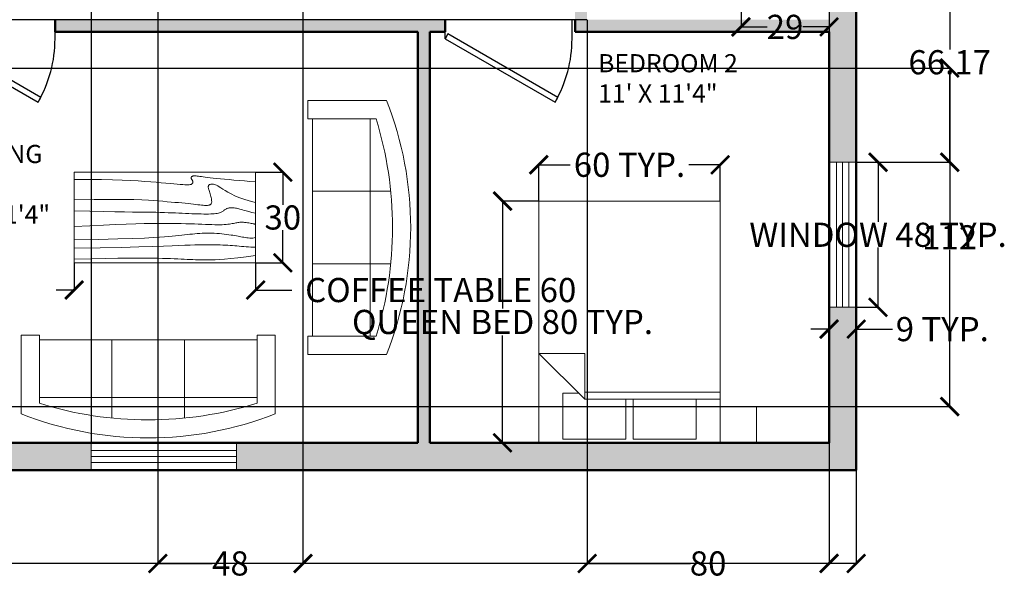
# Model space of a CAD drawing. Units: inches. Extents: x -30 to 744, y -375 to 57.
# Tile 6 of 8: x 355 to 680, y -375 to -190. Entities that reach past the tile are written whole.
import ezdxf

# ---------------------------------------------------------------- set-up
doc = ezdxf.new("R2010")
doc.units = ezdxf.units.IN
doc.header["$MEASUREMENT"] = 0
for name, color, linetype, lineweight in [('A-ANNO-DIMS', 2, 'Continuous', 18), ('A-AREA-IDEN', 7, 'Continuous', 25), ('A-DOOR', 3, 'Continuous', 25), ('A-FURN', 8, 'Continuous', 18), ('A-GLAZ', 4, 'Continuous', 18), ('A-WALL', 7, 'Continuous', 50)]:
    doc.layers.add(name, color=color, linetype=linetype, lineweight=lineweight)
doc.layers.add('A-WALL-PATT', color=251, linetype='Continuous', lineweight=13, true_color=0x636466)
doc.styles.get("Standard").update_dxf_attribs({"font": 'arial.ttf'})
doc.dimstyles.get("Standard").update_dxf_attribs({"dimtxt": 8, "dimasz": 6, "dimexe": 0.18, "dimexo": 0.0625, "dimgap": 0.09, "dimtad": 0, "dimtih": 1, "dimtoh": 1, "dimdec": 0, "dimzin": 0, "dimdsep": 46, "dimlunit": 4, "dimtxsty": 'Standard', "dimblk": 'ARCHTICK', "dimcen": 0.09, "dimadec": 0, "dimazin": 0, "dimtfac": 1, "dimtdec": 0, "dimtofl": 0, "dimtmove": 0, "dimatfit": 1, "dimldrblk": 'ARCHTICK', "dimfxl": 1, "dimtolj": 1, "dimtzin": 0, "dimarcsym": 0})

# ---------------------------------------------------------------- blocks, each defined once
blk = doc.blocks.new('*U4')
for p, q in [((0, 0), (0, 6)), ((40, 0), (40, 6))]:
    blk.add_line(p, q)
blk.add_lwpolyline([(0, 0), (34.64, -20), (35.52, -18.48), (0.87, 1.52)], close=True)
blk.add_arc((0, 0), 40, 330, 0)
blk = doc.blocks.new('*U3')
for p, q in [((0, 0), (0, 6)), ((40, 0), (40, 6))]:
    blk.add_line(p, q)
blk.add_lwpolyline([(0, 0), (34.64, -20), (35.52, -18.48), (0.88, 1.52)], close=True)
blk.add_arc((0, 0), 40, 330, 0)
blk = doc.blocks.new('Bed - Queen')
for p, q in [((0, -80.00003), (0, 0)), ((0, 0), (59.99999, 0)), ((59.99999, 0), (59.99999, -80.00003)), ((7.99999, -1.2), (28.79998, -1.2)), ((7.99999, -14.4), (7.99999, -1.2)), ((28.79998, -1.2), (28.79998, -14.4)), ((31.19999, -1.2), (51.99999, -1.2)), ((31.19999, -14.4), (31.19999, -1.2)), ((51.99999, -1.2), (51.99999, -16.4)), ((0, -14.4), (44.8, -14.4)), ((59.99999, -29.6), (44.8, -14.4)), ((44.8, -14.4), (44.8, -29.6)), ((44.8, -16.8), (0, -16.8)), ((51.99999, -16.4), (46.79936, -16.4)), ((44.8, -29.6), (59.99999, -29.6)), ((59.99999, -80.00003), (0, -80.00003))]:
    blk.add_line(p, q)
blk = doc.blocks.new('Sofa - Roundback 7 ft.')
for p, q in [((-12.00002, -32.4421), (-12.00003, -6.5971)), ((11.99997, -32.4421), (11.99998, -6.5971)), ((-36.000027, -34), (-36.000027, -11.4696)), ((35.99998, -34), (35.99998, -11.4696)), ((-35.999844, -13.3819), (35.9998, -13.3819)), ((-36.000027, -32.4421), (35.99998, -32.4421))]:
    blk.add_line(p, q)
for points in [[(-36.000027, -34), (-42.000027, -34), (-42.000027, -8)], [(41.99998, -8), (41.99998, -34), (35.99998, -34)]]:
    blk.add_lwpolyline(points)
for centre, radius, start, end in [((0, -114.25), 114.25, 68.43141, 111.5686), ((-0.00001, -127.1968), 121.1968, 72.72033, 107.2797)]:
    blk.add_arc(centre, radius, start, end)
blk = doc.blocks.new('Table - Rectangular Woodgrain 60 x 30 in.')
for p, q in [((0, 0), (0, -30)), ((60, 0), (0, 0)), ((60, -30), (60, 0)), ((0, -30), (60, -30))]:
    blk.add_line(p, q)
for points in [[(0, -2.4), (4.8155, -2.418), (9.0302, -2.4688), (12.709, -2.5477), (15.9167, -2.65), (18.7181, -2.7711), (21.1781, -2.9063), (23.3616, -3.0508), (25.3333, -3.2), (27.1477, -3.3495), (28.8172, -3.4958), (30.3437, -3.636), (31.7291, -3.7667), (32.9756, -3.8849), (34.0849, -3.9875), (35.059, -4.0714), (35.9, -4.1334), (36.6114, -4.1711), (37.2041, -4.1854), (37.6906, -4.1779), (38.0833, -4.15), (38.3948, -4.1034), (38.6375, -4.0396), (38.8239, -3.9602), (38.9666, -3.8667), (39.0764, -3.7608), (39.1573, -3.6448), (39.2116, -3.521), (39.2416, -3.3917), (39.2498, -3.2593), (39.2385, -3.1261), (39.21, -2.9944), (39.1666, -2.8667), (39.111, -2.7447), (39.0468, -2.6281), (38.978, -2.5163), (38.9083, -2.4083), (38.8418, -2.3035), (38.7823, -2.201), (38.7337, -2.1001), (38.7, -2), (38.6844, -1.9003), (38.6875, -1.8021), (38.7094, -1.707), (38.75, -1.6167), (38.8094, -1.5326), (38.8875, -1.4563), (38.9844, -1.3893), (39.1, -1.3333), (39.2351, -1.2896), (39.3937, -1.2583), (39.5804, -1.2396), (39.8, -1.2333), (40.057, -1.2396), (40.3562, -1.2583), (40.7023, -1.2896), (41.1, -1.3333), (41.5547, -1.3895), (42.0755, -1.4573), (42.6721, -1.5361), (43.3542, -1.625), (44.1316, -1.7233), (45.014, -1.8302), (46.0114, -1.9449), (47.1333, -2.0667), (48.3862, -2.1947), (49.7625, -2.3281), (51.2513, -2.4663), (52.8416, -2.6083), (54.5226, -2.7535), (56.2833, -2.9011), (58.1127, -3.0501), (60, -3.2)], [(0, -9.2), (6.5759, -9.0858), (11.9385, -9.0365), (16.2527, -9.0418), (19.6833, -9.0917), (22.3952, -9.1759), (24.5531, -9.2844), (26.322, -9.4069), (27.8666, -9.5333), (29.3241, -9.6553), (30.7203, -9.7719), (32.0532, -9.8837), (33.3208, -9.9917), (34.5213, -10.0965), (35.6526, -10.199), (36.7128, -10.2999), (37.7, -10.4), (38.6129, -10.4996), (39.4531, -10.5969), (40.223, -10.6895), (40.925, -10.775), (41.5613, -10.8512), (42.1344, -10.9156), (42.6465, -10.966), (43.1, -11), (43.4976, -11.0158), (43.8437, -11.0136), (44.143, -10.9942), (44.4, -10.9583), (44.6195, -10.9069), (44.8062, -10.8406), (44.9648, -10.7603), (45.1, -10.6667), (45.2155, -10.5598), (45.3114, -10.4365), (45.3871, -10.2929), (45.4416, -10.125), (45.4743, -9.929), (45.4844, -9.7011), (45.4709, -9.4371), (45.4333, -9.1333), (45.3716, -8.7883), (45.2896, -8.4104), (45.1919, -8.0107), (45.0833, -7.6), (44.9685, -7.1893), (44.8521, -6.7896), (44.7388, -6.4117), (44.6333, -6.0667), (44.54, -5.7628), (44.4614, -5.4979), (44.4001, -5.2675), (44.3583, -5.0667), (44.3384, -4.8909), (44.3427, -4.7354), (44.3736, -4.5956), (44.4333, -4.4667), (44.5236, -4.3453), (44.6427, -4.2333), (44.7884, -4.1339), (44.9583, -4.05), (45.1501, -3.9849), (45.3614, -3.9417), (45.59, -3.9234), (45.8333, -3.9333), (46.0915, -3.9749), (46.3734, -4.0531), (46.6906, -4.1736), (47.0542, -4.3417), (47.4756, -4.5629), (47.9661, -4.8427), (48.5372, -5.1866), (49.2, -5.6), (49.9676, -6.0844), (50.8594, -6.625), (51.8965, -7.2031), (53.1, -7.8), (54.491, -8.3969), (56.0906, -8.975), (57.9199, -9.5156), (60, -10)], [(0, -12.8), (5.1847, -12.9322), (9.6213, -13.0323), (13.3963, -13.1059), (16.5958, -13.1583), (19.3063, -13.1952), (21.614, -13.2219), (23.6054, -13.2439), (25.3666, -13.2667), (26.9728, -13.2947), (28.4531, -13.3281), (29.8256, -13.3663), (31.1083, -13.4083), (32.3191, -13.4535), (33.476, -13.501), (34.597, -13.5501), (35.7, -13.6), (36.7984, -13.6497), (37.8875, -13.6979), (38.9578, -13.743), (40, -13.7833), (41.0047, -13.8174), (41.9625, -13.8438), (42.864, -13.8607), (43.7, -13.8667), (44.4631, -13.8604), (45.1552, -13.8417), (45.7801, -13.8104), (46.3416, -13.7667), (46.8439, -13.7104), (47.2906, -13.6417), (47.6858, -13.5604), (48.0333, -13.4667), (48.3375, -13.3608), (48.6042, -13.2448), (48.8396, -13.121), (49.05, -12.9917), (49.2417, -12.8593), (49.4208, -12.7261), (49.5937, -12.5944), (49.7667, -12.4667), (49.9452, -12.3451), (50.1323, -12.2313), (50.3303, -12.1268), (50.5416, -12.0333), (50.7686, -11.9524), (51.0135, -11.8854), (51.2788, -11.8341), (51.5666, -11.8), (51.8785, -11.7843), (52.2116, -11.7865), (52.562, -11.8059), (52.926, -11.8417), (53.2998, -11.8931), (53.6795, -11.9594), (54.0614, -12.0397), (54.4416, -12.1333), (54.8223, -12.2401), (55.2293, -12.3625), (55.6942, -12.5037), (56.2489, -12.6667), (56.9251, -12.8547), (57.7545, -13.0708), (58.7689, -13.3182), (60, -13.6)], [(0, -18), (5.124, -17.7273), (9.6609, -17.5057), (13.6705, -17.3303), (17.2125, -17.1958), (20.3467, -17.0973), (23.1328, -17.0297), (25.6307, -16.9878), (27.9, -16.9667), (29.9928, -16.9617), (31.9302, -16.9703), (33.7254, -16.9907), (35.3917, -17.0208), (36.9423, -17.0588), (38.3906, -17.1026), (39.7499, -17.1503), (41.0333, -17.2), (42.2519, -17.2496), (43.4073, -17.2969), (44.4986, -17.3395), (45.525, -17.375), (46.4858, -17.4012), (47.3802, -17.4156), (48.2074, -17.416), (48.9667, -17.4), (49.6583, -17.3662), (50.2872, -17.3167), (50.8595, -17.2547), (51.3812, -17.1833), (51.8584, -17.1057), (52.2971, -17.025), (52.7034, -16.9443), (53.0833, -16.8667), (53.443, -16.7951), (53.789, -16.7313), (54.128, -16.6768), (54.4666, -16.6334), (54.8115, -16.6024), (55.1693, -16.5854), (55.5465, -16.5841), (55.95, -16.6), (56.3828, -16.6337), (56.8346, -16.6823), (57.2915, -16.7418), (57.7396, -16.8084), (58.165, -16.878), (58.5539, -16.9469), (58.8924, -17.0111), (59.1666, -17.0667), (59.3679, -17.1107), (59.5078, -17.1438), (59.6032, -17.1675), (59.6708, -17.1833), (59.7275, -17.193), (59.7901, -17.1979), (59.8753, -17.1998), (60, -17.2)], [(0, -22.4), (8.0098, -22.2501), (14.4094, -22.1011), (19.4168, -21.9535), (23.25, -21.8083), (26.1269, -21.6663), (28.2656, -21.5281), (29.884, -21.3947), (31.2, -21.2667), (32.3967, -21.1448), (33.5172, -21.0292), (34.5697, -20.9198), (35.5625, -20.8167), (36.5037, -20.7198), (37.4015, -20.6292), (38.2642, -20.5448), (39.1, -20.4667), (39.9164, -20.3951), (40.7187, -20.3313), (41.5117, -20.2768), (42.3, -20.2333), (43.0883, -20.2024), (43.8812, -20.1854), (44.6836, -20.1841), (45.5, -20.2), (46.3328, -20.234), (47.1747, -20.2844), (48.0163, -20.3488), (48.8479, -20.425), (49.66, -20.5106), (50.4429, -20.6031), (51.1872, -20.7004), (51.8833, -20.8), (52.5246, -20.8999), (53.1166, -20.9995), (53.6681, -21.0983), (54.1875, -21.1958), (54.6834, -21.2919), (55.1646, -21.3859), (55.6394, -21.4777), (56.1167, -21.5667), (56.6028, -21.6515), (57.0961, -21.7266), (57.5929, -21.7852), (58.0896, -21.8208), (58.5823, -21.8268), (59.0674, -21.7964), (59.5412, -21.723), (60, -21.6)], [(0, -25.2), (8.6355, -25.0504), (15.7026, -24.9031), (21.4049, -24.7606), (25.9458, -24.625), (29.529, -24.4988), (32.3578, -24.3844), (34.6359, -24.284), (36.5667, -24.2), (38.3213, -24.1341), (39.9417, -24.0854), (41.437, -24.0523), (42.8167, -24.0333), (44.0901, -24.0268), (45.2667, -24.0313), (46.3557, -24.0451), (47.3667, -24.0667), (48.309, -24.0947), (49.1928, -24.1287), (50.0284, -24.168), (50.826, -24.2125), (51.5959, -24.2617), (52.3483, -24.3151), (53.0935, -24.3725), (53.8417, -24.4334), (54.6009, -24.497), (55.3699, -24.561), (56.1454, -24.6226), (56.9239, -24.6792), (57.7021, -24.7279), (58.4764, -24.7662), (59.2435, -24.7911), (60, -24.8)], [(0, -28.8), (5.6867, -28.6681), (10.45, -28.5698), (14.407, -28.5012), (17.675, -28.4584), (20.3711, -28.4374), (22.6125, -28.4344), (24.5164, -28.4455), (26.2, -28.4667), (27.762, -28.4947), (29.2276, -28.5281), (30.6033, -28.5663), (31.8958, -28.6084), (33.1118, -28.6535), (34.2578, -28.7011), (35.3405, -28.7501), (36.3666, -28.8), (37.3443, -28.8497), (38.288, -28.8974), (39.2137, -28.9412), (40.1375, -28.9792), (41.0753, -29.0093), (42.0432, -29.0297), (43.0572, -29.0384), (44.1333, -29.0333), (45.2936, -29.0114), (46.5843, -28.9641), (48.0579, -28.8816), (49.7666, -28.7542), (51.7629, -28.5721), (54.0989, -28.3255), (56.8272, -28.0048), (60, -27.6)]]:
    blk.add_lwpolyline(points)
blk = doc.blocks.new('WIN-48IN')
for p, q in [((0, 0), (0, 48)), ((0, 48), (9, 48)), ((2.5, 48), (2.5, 0)), ((4.5, 48), (4.5, 0)), ((6.5, 48), (6.5, 0)), ((9, 48), (9, 0)), ((9, 48), (9, 0)), ((9, 0), (0, 0))]:
    blk.add_line(p, q)
blk = doc.blocks.new('NIGHTSTAND-12IN')
blk.add_lwpolyline([(0, 12), (0, 0), (12, 0), (12, 12)], close=True)
blk = doc.blocks.new('_ArchTick')
at = {"color": 0, "linetype": 'ByBlock', "const_width": 0.15}
blk.add_lwpolyline([(-0.5, -0.5), (0.5, 0.5)], dxfattribs=at)
blk = doc.blocks.new('*D26')
at = {"layer": 'A-ANNO-DIMS', "color": 0, "lineweight": -2, "transparency": 16777216}
for p, q in [((631.3, -237.46), (638.62, -237.46)), ((638.44, -237.46), (638.44, -257.23)), ((638.44, -285.46), (638.44, -265.69)), ((631.3, -285.46), (638.62, -285.46))]:
    blk.add_line(p, q, dxfattribs=at)
at = {"layer": 'Defpoints', "color": 0, "transparency": 16777216}
for p in [(631.24, -237.46), (638.44, -237.46), (631.24, -285.46)]:
    blk.add_point(p, dxfattribs=at)
at = {"layer": 'A-ANNO-DIMS', "color": 0, "lineweight": -2, "transparency": 16777216, "xscale": 6, "yscale": 6, "zscale": 6}
for p, rotation in [((638.44, -237.46), 90), ((638.44, -285.46), 270)]:
    blk.add_blockref('_ArchTick', p, dxfattribs=dict(at, rotation=rotation))
at = {"layer": 'A-ANNO-DIMS', "color": 0, "transparency": 16777216, "insert": (638.44, -261.46), "char_height": 8, "attachment_point": 5}
blk.add_mtext('\\A1;WINDOW 48 TYP.', dxfattribs=at)
blk = doc.blocks.new('*D27')
at = {"layer": 'A-ANNO-DIMS', "color": 0, "lineweight": -2, "transparency": 16777216}
for p, q in [((622.24, -285.53), (622.24, -292.84)), ((631.24, -285.53), (631.24, -292.84)), ((622.24, -292.66), (616.24, -292.66)), ((631.24, -292.66), (643.24, -292.66))]:
    blk.add_line(p, q, dxfattribs=at)
at = {"layer": 'Defpoints', "color": 0, "transparency": 16777216}
for p in [(622.24, -285.46), (631.24, -285.46), (631.24, -292.66)]:
    blk.add_point(p, dxfattribs=at)
at = {"layer": 'A-ANNO-DIMS', "color": 0, "lineweight": -2, "transparency": 16777216, "xscale": 6, "yscale": 6, "zscale": 6}
blk.add_blockref('_ArchTick', (622.24, -292.66), dxfattribs=at)
at = {"layer": 'A-ANNO-DIMS', "color": 0, "lineweight": -2, "transparency": 16777216, "xscale": 6, "yscale": 6, "zscale": 6, "rotation": 180}
blk.add_blockref('_ArchTick', (631.24, -292.66), dxfattribs=at)
at = {"layer": 'A-ANNO-DIMS', "color": 0, "transparency": 16777216, "insert": (659.69, -292.66), "char_height": 8, "attachment_point": 5}
blk.add_mtext('\\A1;9 TYP.', dxfattribs=at)
blk = doc.blocks.new('*D32')
at = {"layer": 'A-ANNO-DIMS', "color": 0, "lineweight": -2, "transparency": 16777216}
for p, q in [((526.17, -250.3), (514.06, -250.3)), ((514.24, -250.3), (514.24, -285.82)), ((514.24, -330.3), (514.24, -294.77)), ((526.17, -330.3), (514.06, -330.3))]:
    blk.add_line(p, q, dxfattribs=at)
at = {"layer": 'Defpoints', "color": 0, "transparency": 16777216}
for p in [(526.24, -250.3), (514.24, -330.3), (526.24, -330.3)]:
    blk.add_point(p, dxfattribs=at)
at = {"layer": 'A-ANNO-DIMS', "color": 0, "lineweight": -2, "transparency": 16777216, "xscale": 6, "yscale": 6, "zscale": 6}
for p, rotation in [((514.24, -250.3), 90), ((514.24, -330.3), 270)]:
    blk.add_blockref('_ArchTick', p, dxfattribs=dict(at, rotation=rotation))
at = {"layer": 'A-ANNO-DIMS', "color": 0, "transparency": 16777216, "insert": (514.24, -290.3), "char_height": 8, "attachment_point": 5}
blk.add_mtext('\\A1;QUEEN BED 80 TYP.', dxfattribs=at)
blk = doc.blocks.new('*D33')
at = {"layer": 'A-ANNO-DIMS', "color": 0, "lineweight": -2, "transparency": 16777216}
for p, q in [((526.24, -250.23), (526.24, -238.12)), ((526.24, -238.3), (536.65, -238.3)), ((586.24, -238.3), (575.82, -238.3)), ((586.24, -250.23), (586.24, -238.12))]:
    blk.add_line(p, q, dxfattribs=at)
at = {"layer": 'Defpoints', "color": 0, "transparency": 16777216}
for p in [(526.24, -238.3), (526.24, -250.3), (586.24, -250.3)]:
    blk.add_point(p, dxfattribs=at)
at = {"layer": 'A-ANNO-DIMS', "color": 0, "lineweight": -2, "transparency": 16777216, "xscale": 6, "yscale": 6, "zscale": 6, "rotation": 180.0000000000009}
blk.add_blockref('_ArchTick', (526.24, -238.3), dxfattribs=at)
at = {"layer": 'A-ANNO-DIMS', "color": 0, "lineweight": -2, "transparency": 16777216, "xscale": 6, "yscale": 6, "zscale": 6}
blk.add_blockref('_ArchTick', (586.24, -238.3), dxfattribs=at)
at = {"layer": 'A-ANNO-DIMS', "color": 0, "transparency": 16777216, "insert": (556.24, -238.3), "char_height": 8, "attachment_point": 5}
blk.add_mtext('\\A1;60 TYP.', dxfattribs=at)
blk = doc.blocks.new('*D37')
at = {"layer": 'A-ANNO-DIMS', "color": 0, "lineweight": -2, "transparency": 16777216}
for p, q in [((593.12, -185.47), (593.12, -192.86)), ((622.24, -185.47), (622.24, -192.86)), ((593.12, -192.68), (601.78, -192.68)), ((622.24, -192.68), (613.57, -192.68))]:
    blk.add_line(p, q, dxfattribs=at)
at = {"layer": 'Defpoints', "color": 0, "transparency": 16777216}
for p in [(593.12, -185.4), (622.24, -185.4), (622.24, -192.68)]:
    blk.add_point(p, dxfattribs=at)
at = {"layer": 'A-ANNO-DIMS', "color": 0, "lineweight": -2, "transparency": 16777216, "xscale": 6, "yscale": 6, "zscale": 6, "rotation": 180}
blk.add_blockref('_ArchTick', (593.12, -192.68), dxfattribs=at)
at = {"layer": 'A-ANNO-DIMS', "color": 0, "lineweight": -2, "transparency": 16777216, "xscale": 6, "yscale": 6, "zscale": 6}
blk.add_blockref('_ArchTick', (622.24, -192.68), dxfattribs=at)
at = {"layer": 'A-ANNO-DIMS', "color": 0, "transparency": 16777216, "insert": (607.68, -192.68), "char_height": 8, "attachment_point": 5}
blk.add_mtext('\\A1;29', dxfattribs=at)
blk = doc.blocks.new('*D58')
at = {"layer": 'A-ANNO-DIMS', "color": 0, "lineweight": -2, "transparency": 16777216}
for p, q in [((372.57, -270.8), (372.57, -279.92)), ((432.57, -270.8), (432.57, -279.92)), ((372.57, -279.74), (366.57, -279.74)), ((432.57, -279.74), (444.57, -279.74))]:
    blk.add_line(p, q, dxfattribs=at)
at = {"layer": 'Defpoints', "color": 0, "transparency": 16777216}
for p in [(372.57, -270.74), (432.57, -270.74), (432.57, -279.74)]:
    blk.add_point(p, dxfattribs=at)
at = {"layer": 'A-ANNO-DIMS', "color": 0, "lineweight": -2, "transparency": 16777216, "xscale": 6, "yscale": 6, "zscale": 6}
blk.add_blockref('_ArchTick', (372.57, -279.74), dxfattribs=at)
at = {"layer": 'A-ANNO-DIMS', "color": 0, "lineweight": -2, "transparency": 16777216, "xscale": 6, "yscale": 6, "zscale": 6, "rotation": 180}
blk.add_blockref('_ArchTick', (432.57, -279.74), dxfattribs=at)
at = {"layer": 'A-ANNO-DIMS', "color": 0, "transparency": 16777216, "insert": (493.8, -279.74), "char_height": 8, "attachment_point": 5}
blk.add_mtext('\\A1;COFFEE TABLE 60', dxfattribs=at)
blk = doc.blocks.new('*D59')
at = {"layer": 'A-ANNO-DIMS', "color": 0, "lineweight": -2, "transparency": 16777216}
for p, q in [((432.63, -240.74), (441.75, -240.74)), ((441.57, -240.74), (441.57, -251.56)), ((441.57, -270.74), (441.57, -259.91)), ((432.63, -270.74), (441.75, -270.74))]:
    blk.add_line(p, q, dxfattribs=at)
at = {"layer": 'Defpoints', "color": 0, "transparency": 16777216}
for p in [(432.57, -240.74), (441.57, -240.74), (432.57, -270.74)]:
    blk.add_point(p, dxfattribs=at)
at = {"layer": 'A-ANNO-DIMS', "color": 0, "lineweight": -2, "transparency": 16777216, "xscale": 6, "yscale": 6, "zscale": 6}
for p, rotation in [((441.57, -240.74), 90), ((441.57, -270.74), 270)]:
    blk.add_blockref('_ArchTick', p, dxfattribs=dict(at, rotation=rotation))
at = {"layer": 'A-ANNO-DIMS', "color": 0, "transparency": 16777216, "insert": (441.57, -255.74), "char_height": 8, "attachment_point": 5}
blk.add_mtext('\\A1;30', dxfattribs=at)
blk = doc.blocks.new('*D60')
at = {"layer": 'A-ANNO-DIMS', "color": 0, "lineweight": -2, "transparency": 16777216}
for p, q in [((31.24, -339.36), (31.24, -370.38)), ((631.24, -339.36), (631.24, -370.38)), ((31.24, -370.2), (322.3, -370.2)), ((631.24, -370.2), (340.17, -370.2))]:
    blk.add_line(p, q, dxfattribs=at)
at = {"layer": 'Defpoints', "color": 0, "transparency": 16777216}
for p in [(31.24, -339.3), (631.24, -339.3), (631.24, -370.2)]:
    blk.add_point(p, dxfattribs=at)
at = {"layer": 'A-ANNO-DIMS', "color": 0, "lineweight": -2, "transparency": 16777216, "xscale": 6, "yscale": 6, "zscale": 6, "rotation": 180}
blk.add_blockref('_ArchTick', (31.24, -370.2), dxfattribs=at)
at = {"layer": 'A-ANNO-DIMS', "color": 0, "lineweight": -2, "transparency": 16777216, "xscale": 6, "yscale": 6, "zscale": 6}
blk.add_blockref('_ArchTick', (631.24, -370.2), dxfattribs=at)
at = {"layer": 'A-ANNO-DIMS', "color": 0, "transparency": 16777216, "insert": (331.24, -370.2), "char_height": 8, "attachment_point": 5}
blk.add_mtext('\\A1;600', dxfattribs=at)
blk = doc.blocks.new('*D62')
at = {"layer": 'A-ANNO-DIMS', "color": 0, "lineweight": -2, "transparency": 16777216}
for p, q in [((542.24, -190.36), (542.24, -370.38)), ((622.24, -190.36), (622.24, -370.38)), ((542.24, -370.2), (576.42, -370.2)), ((622.24, -370.2), (588.05, -370.2))]:
    blk.add_line(p, q, dxfattribs=at)
at = {"layer": 'Defpoints', "color": 0, "transparency": 16777216}
for p in [(542.24, -190.3), (622.24, -190.3), (622.24, -370.2)]:
    blk.add_point(p, dxfattribs=at)
at = {"layer": 'A-ANNO-DIMS', "color": 0, "lineweight": -2, "transparency": 16777216, "xscale": 6, "yscale": 6, "zscale": 6, "rotation": 180}
blk.add_blockref('_ArchTick', (542.24, -370.2), dxfattribs=at)
at = {"layer": 'A-ANNO-DIMS', "color": 0, "lineweight": -2, "transparency": 16777216, "xscale": 6, "yscale": 6, "zscale": 6}
blk.add_blockref('_ArchTick', (622.24, -370.2), dxfattribs=at)
at = {"layer": 'A-ANNO-DIMS', "color": 0, "transparency": 16777216, "insert": (582.24, -370.2), "char_height": 8, "attachment_point": 5}
blk.add_mtext('\\A1;80', dxfattribs=at)
blk = doc.blocks.new('*D63')
at = {"layer": 'A-ANNO-DIMS', "color": 0, "lineweight": -2, "transparency": 16777216}
for p, q in [((542.17, -132.3), (-16.61, -132.3)), ((-16.43, -132.3), (-16.43, -157.12)), ((-16.43, -190.3), (-16.43, -165.47)), ((542.17, -190.3), (-16.61, -190.3))]:
    blk.add_line(p, q, dxfattribs=at)
at = {"layer": 'Defpoints', "color": 0, "transparency": 16777216}
for p in [(-16.43, -132.3), (542.24, -132.3), (542.24, -190.3)]:
    blk.add_point(p, dxfattribs=at)
at = {"layer": 'A-ANNO-DIMS', "color": 0, "lineweight": -2, "transparency": 16777216, "xscale": 6, "yscale": 6, "zscale": 6}
for p, rotation in [((-16.43, -132.3), 90), ((-16.43, -190.3), 270)]:
    blk.add_blockref('_ArchTick', p, dxfattribs=dict(at, rotation=rotation))
at = {"layer": 'A-ANNO-DIMS', "color": 0, "transparency": 16777216, "insert": (-16.43, -161.3), "char_height": 8, "attachment_point": 5}
blk.add_mtext('\\A1;58', dxfattribs=at)
blk = doc.blocks.new('*D64')
at = {"layer": 'A-ANNO-DIMS', "color": 0, "lineweight": -2, "transparency": 16777216}
for p, q in [((40.3, -206.3), (662.32, -206.3)), ((662.14, -206.3), (662.14, -258.19)), ((662.14, -318.3), (662.14, -266.4)), ((40.3, -318.3), (662.32, -318.3))]:
    blk.add_line(p, q, dxfattribs=at)
at = {"layer": 'Defpoints', "color": 0, "transparency": 16777216}
for p in [(40.24, -206.3), (662.14, -206.3), (40.24, -318.3)]:
    blk.add_point(p, dxfattribs=at)
at = {"layer": 'A-ANNO-DIMS', "color": 0, "lineweight": -2, "transparency": 16777216, "xscale": 6, "yscale": 6, "zscale": 6}
for p, rotation in [((662.14, -206.3), 90), ((662.14, -318.3), 270)]:
    blk.add_blockref('_ArchTick', p, dxfattribs=dict(at, rotation=rotation))
at = {"layer": 'A-ANNO-DIMS', "color": 0, "transparency": 16777216, "insert": (662.14, -262.3), "char_height": 8, "attachment_point": 5}
blk.add_mtext('\\A1;112', dxfattribs=at)
blk = doc.blocks.new('*D74')
at = {"layer": 'A-ANNO-DIMS', "color": 0, "lineweight": -2, "transparency": 16777216}
for p, q in [((318.24, -330.23), (318.24, 51.78)), ((318.24, 51.6), (342.41, 51.6)), ((378.24, 51.6), (354.06, 51.6)), ((378.24, -330.23), (378.24, 51.78))]:
    blk.add_line(p, q, dxfattribs=at)
at = {"layer": 'Defpoints', "color": 0, "transparency": 16777216}
for p in [(378.24, 51.6), (318.24, -330.3), (378.24, -330.3)]:
    blk.add_point(p, dxfattribs=at)
at = {"layer": 'A-ANNO-DIMS', "color": 0, "lineweight": -2, "transparency": 16777216, "xscale": 6, "yscale": 6, "zscale": 6, "rotation": 180}
blk.add_blockref('_ArchTick', (318.24, 51.6), dxfattribs=at)
at = {"layer": 'A-ANNO-DIMS', "color": 0, "lineweight": -2, "transparency": 16777216, "xscale": 6, "yscale": 6, "zscale": 6}
blk.add_blockref('_ArchTick', (378.24, 51.6), dxfattribs=at)
at = {"layer": 'A-ANNO-DIMS', "color": 0, "transparency": 16777216, "insert": (348.24, 51.6), "char_height": 8, "attachment_point": 5}
blk.add_mtext('\\A1;60', dxfattribs=at)
blk = doc.blocks.new('*D78')
at = {"layer": 'A-ANNO-DIMS', "color": 0, "lineweight": -2, "transparency": 16777216}
for p, q in [((631.3, -171.3), (662.32, -171.3)), ((662.14, -171.3), (662.14, -200.21)), ((662.14, -237.46), (662.14, -208.55)), ((631.3, -237.46), (662.32, -237.46))]:
    blk.add_line(p, q, dxfattribs=at)
at = {"layer": 'Defpoints', "color": 0, "transparency": 16777216}
for p in [(631.24, -171.3), (662.14, -171.3), (631.24, -237.46)]:
    blk.add_point(p, dxfattribs=at)
at = {"layer": 'A-ANNO-DIMS', "color": 0, "lineweight": -2, "transparency": 16777216, "xscale": 6, "yscale": 6, "zscale": 6}
for p, rotation in [((662.14, -171.3), 90), ((662.14, -237.46), 270)]:
    blk.add_blockref('_ArchTick', p, dxfattribs=dict(at, rotation=rotation))
at = {"layer": 'A-ANNO-DIMS', "color": 0, "transparency": 16777216, "insert": (662.14, -204.38), "char_height": 8, "attachment_point": 5}
blk.add_mtext('\\A1;66.17', dxfattribs=at)
blk = doc.blocks.new('*D83')
at = {"layer": 'A-ANNO-DIMS', "color": 0, "lineweight": -2, "transparency": 16777216}
for p, q in [((400.24, -132.36), (400.24, -370.38)), ((448.24, -132.36), (448.24, -370.38)), ((400.24, -370.2), (418.25, -370.2)), ((448.24, -370.2), (430.22, -370.2))]:
    blk.add_line(p, q, dxfattribs=at)
at = {"layer": 'Defpoints', "color": 0, "transparency": 16777216}
for p in [(400.24, -132.3), (448.24, -132.3), (448.24, -370.2)]:
    blk.add_point(p, dxfattribs=at)
at = {"layer": 'A-ANNO-DIMS', "color": 0, "lineweight": -2, "transparency": 16777216, "xscale": 6, "yscale": 6, "zscale": 6, "rotation": 180}
blk.add_blockref('_ArchTick', (400.24, -370.2), dxfattribs=at)
at = {"layer": 'A-ANNO-DIMS', "color": 0, "lineweight": -2, "transparency": 16777216, "xscale": 6, "yscale": 6, "zscale": 6}
blk.add_blockref('_ArchTick', (448.24, -370.2), dxfattribs=at)
at = {"layer": 'A-ANNO-DIMS', "color": 0, "transparency": 16777216, "insert": (424.24, -370.2), "char_height": 8, "attachment_point": 5}
blk.add_mtext('\\A1;48', dxfattribs=at)

msp = doc.modelspace()

# ---------------------------------------------------------------- hatches: boundary and pattern name
at = {"layer": 'A-WALL-PATT'}
h = msp.add_hatch(color=256, dxfattribs=at)
h.dxf.hatch_style = 1
h.paths.add_polyline_path([(40.2356, 11.7031), (204.2356, 11.7031), (204.2356, -24.2969), (208.2356, -24.2969), (208.2356, 11.7031), (233.4275, 11.7031), (233.4275, 20.7031), (31.2356, 20.7031), (31.2356, -34.2969), (40.2356, -34.2969)])
h.paths.add_polyline_path([(40.2356, -82.2969), (31.2356, -82.2969), (31.2356, -132.2969), (40.2356, -132.2969), (51.0767, -132.2969), (111.3137, -132.2969), (111.3137, -143.2969), (120.3137, -143.2969), (120.3137, -132.2969), (156.2356, -132.2969), (156.2356, -128.2969), (113.6001, -128.2969), (113.6001, -128.3034), (53.6001, -128.3034), (40.2356, -128.2969)])
h.paths.add_polyline_path([(302.4681, 20.7031), (257.4275, 20.7031), (257.4275, 11.7031), (286.2356, 11.7031), (286.2356, -60.2969), (208.2356, -60.2969), (208.2356, -54.2969), (204.2356, -54.2969), (204.2356, -64.2969), (208.2356, -64.2969), (286.2356, -64.2969), (286.2356, -128.2969), (264.8954, -128.2969), (208.2356, -128.2969), (204.2356, -128.2969), (198.2356, -128.2969), (198.2356, -132.2969), (290.2356, -132.2969), (290.2356, -128.2969), (290.2356, 11.7031), (302.4681, 11.7031)])
h.paths.add_polyline_path([(405.515, 20.7031), (350.4681, 20.7031), (350.4681, 11.7031), (362.2356, 11.7031), (362.2356, -34.2969), (366.2356, -34.2969), (366.2356, 11.7031), (405.515, 11.7031)])
h.paths.add_polyline_path([(530.2713, 20.7031), (453.515, 20.7031), (453.515, 11.7031), (486.2356, 11.7031), (486.2356, -128.2969), (448.2356, -128.2969), (448.2356, -132.2969), (486.2356, -132.2969), (490.2356, -132.2969), (496.2356, -132.2969), (496.2356, -128.2969), (490.2356, -128.2969), (490.2356, 11.7031), (530.2713, 11.7031)])
h.paths.add_polyline_path([(631.2356, 20.7031), (578.2713, 20.7031), (578.2713, 11.7031), (622.2356, 11.7031), (622.2356, -37.4001), (631.2356, -37.4001)])
h.paths.add_polyline_path([(631.2356, -85.4001), (622.2356, -85.4001), (622.2356, -91.4001), (622.2356, -103.4001), (622.2356, -128.2969), (538.2356, -128.2969), (538.2356, -132.2969), (538.2356, -154.2969), (542.2356, -154.2969), (542.2356, -132.2969), (575.1375, -132.2969), (585.6313, -131.9348), (585.6438, -132.2969), (622.2356, -132.2969), (622.2356, -147.2969), (631.2356, -147.2969)])
h.paths.add_polyline_path([(631.2356, -171.2969), (622.2356, -171.2969), (622.2356, -185.4028), (622.2356, -186.2969), (622.2356, -190.2969), (542.2356, -190.2969), (542.2356, -184.2969), (538.2356, -184.2969), (538.2356, -190.2969), (538.2356, -194.2969), (622.2356, -194.2969), (622.2356, -237.4632), (631.2356, -237.4632)])
h.paths.add_polyline_path([(631.2356, -285.4632), (622.2356, -285.4632), (622.2356, -330.2969), (490.2356, -330.2969), (490.2356, -194.2969), (494.2356, -194.2969), (495.2356, -194.2969), (495.2356, -190.2969), (494.2356, -190.2969), (490.2356, -190.2969), (486.2356, -190.2969), (366.2356, -190.2969), (366.2356, -194.2969), (486.2356, -194.2969), (486.2356, -330.2969), (426.2356, -330.2969), (426.2356, -339.2969), (631.2356, -339.2969)])
h.paths.add_polyline_path([(378.2356, -330.2969), (318.2356, -330.2969), (318.2356, -194.2969), (324.2356, -194.2969), (324.2356, -190.2969), (318.2356, -190.2969), (314.2356, -190.2969), (314.2356, -194.2969), (314.2356, -330.2969), (278.2356, -330.2969), (278.2356, -339.2969), (378.2356, -339.2969)])
h.paths.add_polyline_path([(190.2356, -330.2969), (40.2356, -330.2969), (40.2356, -318.2969), (31.2356, -318.2969), (31.2356, -330.2969), (31.2356, -339.2969), (190.2356, -339.2969)])
h.paths.add_polyline_path([(230.2356, -330.2969), (194.2356, -330.2969), (194.2356, -194.2969), (194.2356, -190.2969), (190.2356, -190.2969), (184.2356, -190.2969), (184.2356, -194.2969), (190.2356, -194.2969), (190.2356, -339.2969), (230.2356, -339.2969)])
h.paths.add_polyline_path([(142.2356, -190.2969), (120.3137, -190.2969), (120.3137, -184.2969), (116.3137, -184.2969), (111.3137, -184.2969), (111.3137, -190.2969), (40.2356, -190.2969), (31.2356, -190.2969), (31.2356, -194.2969), (31.2356, -206.2969), (40.2356, -206.2969), (40.2356, -194.2969), (142.2356, -194.2969)])

# ---------------------------------------------------------------- linework, layer by layer
at = {"layer": 'A-WALL'}
for p, q in [((366.2356, -190.2969), (366.2356, -194.2969)), ((495.2356, -190.2969), (495.2356, -194.2969)), ((538.2356, -190.2969), (538.2356, -194.2969)), ((366.2356, -194.2969), (486.2356, -194.2969)), ((486.2356, -194.2969), (486.2356, -330.2969)), ((490.2356, -194.2969), (494.2356, -194.2969)), ((490.2356, -194.3643), (490.2356, -330.2969)), ((495.2356, -194.2969), (494.2356, -194.2969)), ((622.2356, -194.2969), (538.2356, -194.2969)), ((622.2356, -194.2969), (622.2356, -330.2969)), ((486.2356, -330.2969), (318.2356, -330.2969)), ((622.2356, -330.2969), (490.2356, -330.2969))]:
    msp.add_line(p, q, dxfattribs=at)
msp.add_lwpolyline([(31.2356, -132.2969), (31.2356, 20.7031), (631.2356, 20.7031), (631.2356, -339.2969), (190.2356, -339.2969)], dxfattribs=at)

# ---------------------------------------------------------------- block references
at = {"layer": 'A-DOOR', "xscale": 1.05, "yscale": 1.05, "zscale": 1.05}
for name, p in [('*U4', (324.2356, -196.5969)), ('*U3', (495.2356, -196.5969))]:
    msp.add_blockref(name, p, dxfattribs=at)
at = {"layer": 'A-FURN'}
for name, p, rotation in [('Sofa - Roundback 7 ft.', (483.8654, -259.0482), 270), ('Bed - Queen', (586.2356, -330.2969), 180.0000000000009), ('Sofa - Roundback 7 ft.', (397.0373, -328.6834), 180), ('NIGHTSTAND-12IN', (514.2357, -318.2973), 270.0000000000007), ('NIGHTSTAND-12IN', (586.2357, -318.2973), 270.0000000000007)]:
    msp.add_blockref(name, p, dxfattribs=dict(at, rotation=rotation))
msp.add_blockref('Table - Rectangular Woodgrain 60 x 30 in.', (372.5661, -240.7371), dxfattribs=at)
at = {"layer": 'A-GLAZ'}
msp.add_blockref('WIN-48IN', (622.236, -285.4631), dxfattribs=at)
at = {"layer": 'A-GLAZ', "rotation": 270}
msp.add_blockref('WIN-48IN', (378.2357, -330.2973), dxfattribs=at)

# ---------------------------------------------------------------- texts
at = {"layer": 'A-AREA-IDEN', "char_height": 6, "attachment_point": 1}
for s, width, insert in [('BEDROOM 2\\P11\' X 11\'4"', 68.664679, (545.8607, -201.6961)), ('DRAWING ROOM \\P14\' X 11\'4"', 61.140655, (325.0959, -231.7288))]:
    msp.add_mtext_dynamic_manual_height_columns(s, width=width, gutter_width=1, heights=[0], dxfattribs=dict(at, insert=insert))

# ---------------------------------------------------------------- dimensions: what is measured, and where the dimension line sits
at = {"layer": 'A-ANNO-DIMS'}
for base, p1, p2, picture, middle in [((378.2356, 51.6031), (318.2356, -330.2969), (378.2356, -330.2969), '*D74', (348.2356, 51.6031)), ((448.2356, -370.1969), (400.2356, -132.2969), (448.2356, -132.2969), '*D83', (424.2356, -370.1969)), ((622.2356, -192.6828), (593.1157, -185.4028), (622.2356, -185.4028), '*D37', (607.6756, -192.6828)), ((622.2356, -370.1969), (542.2356, -190.2969), (622.2356, -190.2969), '*D62', (582.2356, -370.1969)), ((631.2356, -370.1969), (31.2356, -339.2969), (631.2356, -339.2969), '*D60', (331.2356, -370.1969))]:
    dim = msp.add_linear_dim(base=base, p1=p1, p2=p2, dimstyle='Standard', override={"dimdec": 0, "dimlfac": 1, "dimrnd": 0, "dimzin": 0, "dimdsep": 46, "dimlunit": 2}, dxfattribs=at)
    dim.commit()
    dim.dimension.update_dxf_attribs({"geometry": picture, "text_midpoint": middle})
for base, p1, p2, override, picture, middle in [((-16.4253, -132.2969), (542.2356, -190.2969), (542.2356, -132.2969), {"dimdec": 0, "dimlfac": 1, "dimrnd": 0, "dimzin": 0, "dimdsep": 46, "dimlunit": 2}, '*D63', (-16.4253, -161.2969)), ((662.1356, -171.2969), (631.2356, -237.4632), (631.2356, -171.2969), {"dimdec": 2, "dimlfac": 1, "dimrnd": 0, "dimzin": 0, "dimdsep": 46, "dimlunit": 2}, '*D78', (662.1356, -204.38)), ((662.1356, -206.2969), (40.2356, -318.2969), (40.2356, -206.2969), {"dimdec": 0, "dimlfac": 1, "dimrnd": 0, "dimzin": 0, "dimdsep": 46, "dimlunit": 2}, '*D64', (662.1356, -262.2969)), ((441.5661, -240.7371), (432.5661, -270.7371), (432.5661, -240.7371), {"dimdec": 0, "dimlfac": 1, "dimrnd": 0, "dimzin": 0, "dimdsep": 46, "dimlunit": 2}, '*D59', (441.5661, -255.7371))]:
    dim = msp.add_linear_dim(base=base, p1=p1, p2=p2, angle=90, dimstyle='Standard', override=override, dxfattribs=at)
    dim.commit()
    dim.dimension.update_dxf_attribs({"geometry": picture, "text_midpoint": middle})
for base, p1, p2, angle, text, picture, middle in [((526.2356, -238.2968), (586.2356, -250.2968), (526.2356, -250.2968), 180, '<> TYP.', '*D33', (556.2356, -238.2968)), ((638.4356, -237.4632), (631.2356, -285.4632), (631.2356, -237.4632), 90, 'WINDOW <> TYP.', '*D26', (638.4356, -261.4632)), ((514.2356, -330.2969), (526.2356, -250.2968), (526.2356, -330.2969), 270, 'QUEEN BED <> TYP.', '*D32', (514.2356, -290.2969))]:
    dim = msp.add_linear_dim(base=base, p1=p1, p2=p2, angle=angle, text=text, dimstyle='Standard', override={"dimdec": 0, "dimlfac": 1, "dimrnd": 0, "dimzin": 0, "dimdsep": 46, "dimlunit": 2}, dxfattribs=at)
    dim.commit()
    dim.dimension.update_dxf_attribs({"geometry": picture, "text_midpoint": middle})
for base, p1, p2, text, picture, middle in [((432.5661, -279.7371), (372.5661, -270.7371), (432.5661, -270.7371), 'COFFEE TABLE <>', '*D58', (493.7966, -279.7371)), ((631.2356, -292.6632), (622.2356, -285.4632), (631.2356, -285.4632), '<> TYP.', '*D27', (659.6885, -292.6632))]:
    dim = msp.add_linear_dim(base=base, p1=p1, p2=p2, text=text, dimstyle='Standard', override={"dimdec": 0, "dimlfac": 1, "dimrnd": 0, "dimzin": 0, "dimdsep": 46, "dimlunit": 2}, dxfattribs=at)
    dim.commit()
    dim.dimension.update_dxf_attribs({"geometry": picture, "text_midpoint": middle})

doc.saveas('drawing.dxf')
